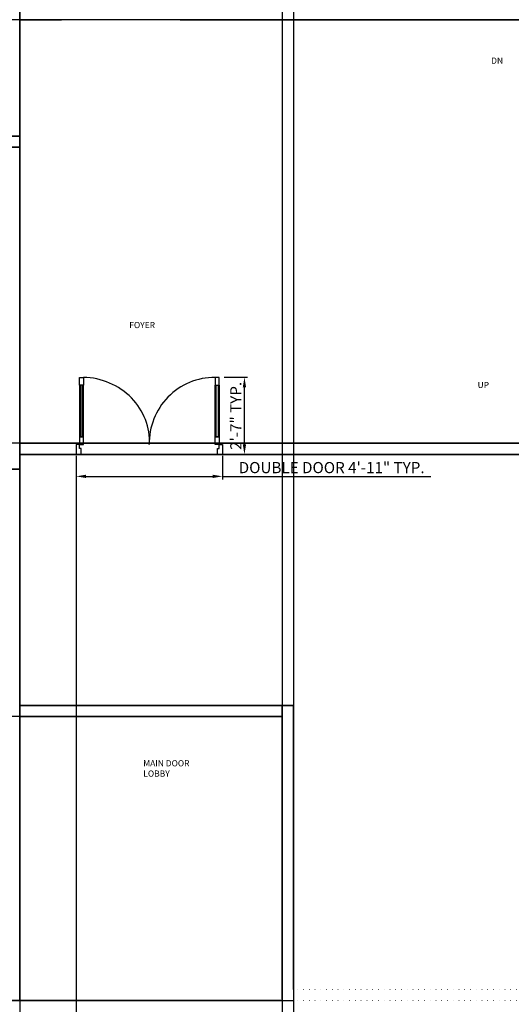
# Model space of a CAD drawing. Units: inches. Extents: x 1239 to 2276906, y 2273 to 321338.
# Tile 11 of 23: x 1556 to 1754, y 2629 to 3026. Entities that reach past the tile are written whole.
import ezdxf

# ---------------------------------------------------------------- set-up
doc = ezdxf.new("R2010")
doc.units = ezdxf.units.IN
doc.linetypes.add('DOT', pattern=[6.35, 0, -6.35])
for name, color, linetype, lineweight in [('A-ANNO-DIMS', 2, 'Continuous', 18), ('A-ANNO-TEXT', 7, 'Continuous', 18), ('A-AREA-IDEN', 7, 'Continuous', 18), ('A-FLOR-PORCH', 7, 'Continuous', 25), ('BEAM LINE', 4, 'DOT', 18), ('DOOR', 1, 'Continuous', 25), ('wall', 7, 'Continuous', 35)]:
    doc.layers.add(name, color=color, linetype=linetype, lineweight=lineweight)
doc.styles.get("Standard").update_dxf_attribs({"font": 'arial.ttf'})
doc.dimstyles.new('ISO-25', dxfattribs={"dimtxt": 4.5, "dimasz": 4, "dimexe": 1.25, "dimexo": 0.625, "dimtad": 1, "dimdec": 1, "dimlunit": 3, "dimtxsty": 'Standard', "dimcen": 2.5, "dimadec": 0, "dimazin": 0, "dimtfac": 1, "dimtdec": 1, "dimtmove": 0, "dimatfit": 3, "dimfxl": 1, "dimarcsym": 0})

# ---------------------------------------------------------------- blocks, each defined once
blk = doc.blocks.new('DOOR-DOUBLE-60')
for p, q in [((1.38, 27.95), (1.38, 31.1)), ((1.38, 31.1), (2.95, 31.1)), ((1.38, 27.95), (1.38, 7.09)), ((2.95, 27.95), (1.38, 27.95)), ((2.95, 27.95), (1.38, 27.95)), ((1.77, 27.95), (1.77, 7.09)), ((2.56, 27.95), (1.77, 27.95)), ((2.56, 7.09), (2.56, 27.95)), ((2.95, 31.1), (2.95, 27.95)), ((2.95, 7.09), (2.95, 27.95)), ((56.1, 31.1), (56.1, 27.95)), ((57.68, 31.1), (56.1, 31.1)), ((56.1, 27.95), (57.68, 27.95)), ((56.1, 7.09), (56.1, 27.95)), ((56.1, 27.95), (57.68, 27.95)), ((56.5, 7.09), (56.5, 27.95)), ((56.5, 27.95), (57.28, 27.95)), ((57.28, 27.95), (57.28, 7.09)), ((57.68, 27.95), (57.68, 31.1)), ((57.68, 27.95), (57.68, 7.09)), ((1.38, 7.09), (1.38, 3.94)), ((2.95, 7.09), (1.38, 7.09)), ((1.38, 7.09), (2.95, 7.09)), ((1.77, 7.09), (2.56, 7.09)), ((2.95, 3.94), (2.95, 7.09)), ((57.68, 7.09), (56.1, 7.09)), ((56.1, 3.94), (56.1, 7.09)), ((56.1, 7.09), (57.68, 7.09)), ((57.28, 7.09), (56.5, 7.09)), ((57.68, 7.09), (57.68, 3.94)), ((0, 3.94), (0, 0)), ((1.38, 3.94), (0, 3.94)), ((0, 0), (1.97, 0)), ((1.38, 3.94), (2.95, 3.94)), ((1.38, 2.36), (1.38, 3.94)), ((1.97, 2.36), (1.38, 2.36)), ((1.97, 1.97), (1.97, 2.36)), ((1.97, 0), (1.97, 1.97)), ((57.68, 3.94), (56.1, 3.94)), ((57.09, 1.97), (57.09, 2.36)), ((57.09, 2.36), (57.68, 2.36)), ((57.09, 0), (57.09, 1.97)), ((59.06, 0), (57.09, 0)), ((57.68, 3.94), (59.06, 3.94)), ((57.68, 2.36), (57.68, 3.94)), ((59.06, 3.94), (59.06, 0))]:
    blk.add_line(p, q)
blk.add_arc((55.99, 4.6), 26.5, 89.7657, 181.4438)
blk.add_ellipse((2.91, 5.95), major_axis=(26.26, -4.79), ratio=0.940794, start_param=0.11153, end_param=1.73917)
blk = doc.blocks.new('*D52')
at = {"layer": 'A-ANNO-DIMS', "color": 0, "lineweight": -2, "transparency": 16777216}
for p, q in [((1578.7, 2850.27), (1578.7, 2840.79)), ((1637.76, 2850.27), (1637.76, 2840.79)), ((1582.7, 2842.04), (1633.76, 2842.04)), ((1637.76, 2842.04), (1721.91, 2842.04))]:
    blk.add_line(p, q, dxfattribs=at)
at = {"layer": 'A-ANNO-DIMS', "color": 0, "transparency": 16777216}
for points in [[(1582.7, 2842.71), (1582.7, 2841.37), (1578.7, 2842.04)], [(1633.76, 2842.71), (1633.76, 2841.37), (1637.76, 2842.04)]]:
    blk.add_solid(points, dxfattribs=at)
at = {"layer": 'Defpoints', "color": 0, "transparency": 16777216}
for p in [(1578.7, 2850.9), (1637.76, 2850.9), (1637.76, 2842.04)]:
    blk.add_point(p, dxfattribs=at)
at = {"layer": 'A-ANNO-DIMS', "color": 0, "transparency": 16777216, "insert": (1681.83, 2844.99), "char_height": 4.5, "attachment_point": 5}
blk.add_mtext('DOUBLE DOOR 4\'-11" TYP.', dxfattribs=at)
blk = doc.blocks.new('*D53')
at = {"layer": 'A-ANNO-DIMS', "color": 0, "lineweight": -2, "transparency": 16777216}
for p, q in [((1638.38, 2882.03), (1647.86, 2882.03)), ((1646.61, 2854.9), (1646.61, 2878.03)), ((1638.38, 2850.9), (1647.86, 2850.9))]:
    blk.add_line(p, q, dxfattribs=at)
at = {"layer": 'A-ANNO-DIMS', "color": 0, "transparency": 16777216}
for points in [[(1645.95, 2878.03), (1647.28, 2878.03), (1646.61, 2882.03)], [(1645.95, 2854.9), (1647.28, 2854.9), (1646.61, 2850.9)]]:
    blk.add_solid(points, dxfattribs=at)
at = {"layer": 'Defpoints', "color": 0, "transparency": 16777216}
for p in [(1637.76, 2882.03), (1646.61, 2882.03), (1637.76, 2850.9)]:
    blk.add_point(p, dxfattribs=at)
at = {"layer": 'A-ANNO-DIMS', "color": 0, "transparency": 16777216, "insert": (1643.73, 2866.46), "char_height": 4.5, "attachment_point": 5, "rotation": 90}
blk.add_mtext('2\'-7" TYP.', dxfattribs=at)
blk = doc.blocks.new('*D87')
at = {"layer": 'A-ANNO-DIMS', "color": 0, "lineweight": -2, "transparency": 16777216}
for p, q in [((1666.38, 3250.77), (1666.38, 2275.7)), ((1921.38, 3250.77), (1921.38, 2275.7)), ((1670.38, 2276.95), (1917.38, 2276.95))]:
    blk.add_line(p, q, dxfattribs=at)
at = {"layer": 'A-ANNO-DIMS', "color": 0, "transparency": 16777216}
for points in [[(1670.38, 2277.61), (1670.38, 2276.28), (1666.38, 2276.95)], [(1917.38, 2277.61), (1917.38, 2276.28), (1921.38, 2276.95)]]:
    blk.add_solid(points, dxfattribs=at)
at = {"layer": 'Defpoints', "color": 0, "transparency": 16777216}
for p in [(1666.38, 3251.4), (1921.38, 3251.4), (1921.38, 2276.95)]:
    blk.add_point(p, dxfattribs=at)
at = {"layer": 'A-ANNO-DIMS', "color": 0, "transparency": 16777216, "insert": (1793.88, 2279.87), "char_height": 4.5, "attachment_point": 5}
blk.add_mtext('21\'-3"', dxfattribs=at)
blk = doc.blocks.new('*D96')
at = {"layer": 'A-ANNO-DIMS', "color": 0, "lineweight": -2, "transparency": 16777216}
for p, q in [((1555.88, 2629.77), (1555.88, 2275.7)), ((1661.88, 2629.77), (1661.88, 2275.7)), ((1559.88, 2276.95), (1657.88, 2276.95))]:
    blk.add_line(p, q, dxfattribs=at)
at = {"layer": 'A-ANNO-DIMS', "color": 0, "transparency": 16777216}
for points in [[(1559.88, 2277.61), (1559.88, 2276.28), (1555.88, 2276.95)], [(1657.88, 2277.61), (1657.88, 2276.28), (1661.88, 2276.95)]]:
    blk.add_solid(points, dxfattribs=at)
at = {"layer": 'Defpoints', "color": 0, "transparency": 16777216}
for p in [(1555.88, 2630.4), (1661.88, 2630.4), (1661.88, 2276.95)]:
    blk.add_point(p, dxfattribs=at)
at = {"layer": 'A-ANNO-DIMS', "color": 0, "transparency": 16777216, "insert": (1608.88, 2279.87), "char_height": 4.5, "attachment_point": 5}
blk.add_mtext('8\'-10"', dxfattribs=at)
blk = doc.blocks.new('*D97')
at = {"layer": 'A-ANNO-DIMS', "color": 0, "lineweight": -2, "transparency": 16777216}
for p, q in [((1661.26, 2745.04), (1247.33, 2745.04)), ((1248.58, 2634.4), (1248.58, 2741.04)), ((1661.26, 2630.4), (1247.33, 2630.4))]:
    blk.add_line(p, q, dxfattribs=at)
at = {"layer": 'A-ANNO-DIMS', "color": 0, "transparency": 16777216}
for points in [[(1247.92, 2741.04), (1249.25, 2741.04), (1248.58, 2745.04)], [(1247.92, 2634.4), (1249.25, 2634.4), (1248.58, 2630.4)]]:
    blk.add_solid(points, dxfattribs=at)
at = {"layer": 'Defpoints', "color": 0, "transparency": 16777216}
for p in [(1248.58, 2745.04), (1661.88, 2745.04), (1661.88, 2630.4)]:
    blk.add_point(p, dxfattribs=at)
at = {"layer": 'A-ANNO-DIMS', "color": 0, "transparency": 16777216, "insert": (1245.63, 2687.72), "char_height": 4.5, "attachment_point": 5, "rotation": 90}
blk.add_mtext('9\'-6 1/2"', dxfattribs=at)
blk = doc.blocks.new('*D98')
at = {"layer": 'A-ANNO-DIMS', "color": 0, "lineweight": -2, "transparency": 16777216}
for p, q in [((1772.76, 3026.4), (1247.33, 3026.4)), ((1248.58, 2859.4), (1248.58, 3022.4)), ((1772.76, 2855.4), (1247.33, 2855.4))]:
    blk.add_line(p, q, dxfattribs=at)
at = {"layer": 'A-ANNO-DIMS', "color": 0, "transparency": 16777216}
for points in [[(1247.92, 3022.4), (1249.25, 3022.4), (1248.58, 3026.4)], [(1247.92, 2859.4), (1249.25, 2859.4), (1248.58, 2855.4)]]:
    blk.add_solid(points, dxfattribs=at)
at = {"layer": 'Defpoints', "color": 0, "transparency": 16777216}
for p in [(1248.58, 3026.4), (1773.38, 3026.4), (1773.38, 2855.4)]:
    blk.add_point(p, dxfattribs=at)
at = {"layer": 'A-ANNO-DIMS', "color": 0, "transparency": 16777216, "insert": (1245.66, 2940.9), "char_height": 4.5, "attachment_point": 5, "rotation": 90}
blk.add_mtext('14\'-3"', dxfattribs=at)
blk = doc.blocks.new('*D111')
at = {"layer": 'A-ANNO-DIMS', "color": 0, "lineweight": -2, "transparency": 16777216}
for p, q in [((1547.38, 3607.7), (1543.38, 3607.7)), ((1551.38, 2635.52), (1551.38, 3608.95)), ((1551.38, 3607.7), (1555.88, 3607.7)), ((1555.88, 2631.02), (1555.88, 3608.95)), ((1559.88, 3607.7), (1587.58, 3607.7))]:
    blk.add_line(p, q, dxfattribs=at)
at = {"layer": 'A-ANNO-DIMS', "color": 0, "transparency": 16777216}
for points in [[(1547.38, 3608.36), (1547.38, 3607.03), (1551.38, 3607.7)], [(1559.88, 3608.36), (1559.88, 3607.03), (1555.88, 3607.7)]]:
    blk.add_solid(points, dxfattribs=at)
at = {"layer": 'Defpoints', "color": 0, "transparency": 16777216}
for p in [(1555.88, 3607.7), (1551.38, 2634.9), (1555.88, 2630.4)]:
    blk.add_point(p, dxfattribs=at)
at = {"layer": 'A-ANNO-DIMS', "color": 0, "transparency": 16777216, "insert": (1575.73, 3610.65), "char_height": 4.5, "attachment_point": 5}
blk.add_mtext('0\'-4 1/2"', dxfattribs=at)
blk = doc.blocks.new('*D112')
at = {"layer": 'A-ANNO-DIMS', "color": 0, "lineweight": -2, "transparency": 16777216}
for p, q in [((1555.88, 3371.77), (1555.88, 2275.7)), ((1661.88, 3371.77), (1661.88, 2275.7)), ((1559.88, 2276.95), (1657.88, 2276.95))]:
    blk.add_line(p, q, dxfattribs=at)
at = {"layer": 'A-ANNO-DIMS', "color": 0, "transparency": 16777216}
for points in [[(1559.88, 2277.61), (1559.88, 2276.28), (1555.88, 2276.95)], [(1657.88, 2277.61), (1657.88, 2276.28), (1661.88, 2276.95)]]:
    blk.add_solid(points, dxfattribs=at)
at = {"layer": 'Defpoints', "color": 0, "transparency": 16777216}
for p in [(1555.88, 3372.4), (1661.88, 3372.4), (1661.88, 2276.95)]:
    blk.add_point(p, dxfattribs=at)
at = {"layer": 'A-ANNO-DIMS', "color": 0, "transparency": 16777216, "insert": (1608.88, 2279.87), "char_height": 4.5, "attachment_point": 5}
blk.add_mtext('8\'-10"', dxfattribs=at)
blk = doc.blocks.new('*D114')
at = {"layer": 'A-ANNO-DIMS', "color": 0, "lineweight": -2, "transparency": 16777216}
for p, q in [((1555.88, 2850.27), (1555.88, 2275.7)), ((1578.7, 2850.27), (1578.7, 2275.7)), ((1559.88, 2276.95), (1574.7, 2276.95))]:
    blk.add_line(p, q, dxfattribs=at)
at = {"layer": 'A-ANNO-DIMS', "color": 0, "transparency": 16777216}
for points in [[(1559.88, 2277.61), (1559.88, 2276.28), (1555.88, 2276.95)], [(1574.7, 2277.61), (1574.7, 2276.28), (1578.7, 2276.95)]]:
    blk.add_solid(points, dxfattribs=at)
at = {"layer": 'Defpoints', "color": 0, "transparency": 16777216}
for p in [(1555.88, 2850.9), (1578.7, 2850.9), (1578.7, 2276.95)]:
    blk.add_point(p, dxfattribs=at)
at = {"layer": 'A-ANNO-DIMS', "color": 0, "transparency": 16777216, "insert": (1567.29, 2279.83), "char_height": 4.5, "attachment_point": 5}
blk.add_mtext('1\'-11"', dxfattribs=at)

msp = doc.modelspace()

# ---------------------------------------------------------------- linework, layer by layer
at = {"layer": 'A-FLOR-PORCH'}
msp.add_lwpolyline([(1551.38, 2630.4), (1666.38, 2630.4), (1666.38, 2555.13), (1551.38, 2555.13)], close=True, dxfattribs=at)
at = {"layer": 'BEAM LINE', "ltscale": 0.35}
for p, q in [((1921.38, 2634.9), (1666.38, 2634.9)), ((1921.38, 2630.4), (1661.88, 2630.4))]:
    msp.add_line(p, q, dxfattribs=at)
at = {"layer": 'wall'}
for p, q in [((1555.88, 3069.4), (1555.88, 2855.4)), ((1572.71, 3026.4), (1555.88, 3026.4)), ((1773.38, 3026.4), (1620.71, 3026.4)), ((1555.88, 2979.4), (1359.38, 2979.4)), ((1555.88, 2974.9), (1359.38, 2974.9)), ((1773.38, 2855.4), (1555.88, 2855.4)), ((1921.38, 2855.4), (1666.38, 2855.4)), ((1661.88, 2850.9), (1555.88, 2850.9)), ((1555.88, 2850.9), (1555.88, 2630.4)), ((1661.88, 2850.9), (1666.38, 2850.9)), ((1921.38, 2850.9), (1666.38, 2850.9)), ((1555.88, 2844.9), (1551.38, 2844.9)), ((1661.88, 2749.54), (1555.88, 2749.54)), ((1661.88, 2749.54), (1661.88, 2630.4)), ((1661.88, 2749.54), (1666.38, 2749.54)), ((1666.38, 2749.54), (1666.38, 2634.9)), ((1661.88, 2745.04), (1555.88, 2745.04)), ((1555.88, 2630.4), (1359.38, 2630.4))]:
    msp.add_line(p, q, dxfattribs=at)

# ---------------------------------------------------------------- block references
at = {"layer": 'DOOR'}
msp.add_blockref('DOOR-DOUBLE-60', (1578.7, 2850.9), dxfattribs=at)

# ---------------------------------------------------------------- texts
at = {"layer": 'A-ANNO-TEXT', "char_height": 2.5, "attachment_point": 1}
for s, insert in [('DN ', (1746.22, 3011.12)), ('UP', (1740.74, 2880.18))]:
    msp.add_mtext_dynamic_manual_height_columns(s, width=44.9462, gutter_width=12.5, heights=[0], dxfattribs=dict(at, insert=insert))
at = {"layer": 'A-AREA-IDEN', "char_height": 2.5, "attachment_point": 1}
for s, insert in [('FOYER', (1600.12, 2904.38)), ('MAIN DOOR\\PLOBBY', (1605.79, 2727.46))]:
    msp.add_mtext_dynamic_manual_height_columns(s, width=44.9462, gutter_width=12.5, heights=[0], dxfattribs=dict(at, insert=insert))

# ---------------------------------------------------------------- dimensions: what is measured, and where the dimension line sits
at = {"layer": 'A-ANNO-DIMS'}
for base, p1, p2, picture, middle in [((1555.88, 3607.7), (1551.38, 2634.9), (1555.88, 2630.4), '*D111', (1575.73, 3610.65)), ((1661.88, 2276.95), (1555.88, 3372.4), (1661.88, 3372.4), '*D112', (1608.88, 2279.87)), ((1921.38, 2276.95), (1666.38, 3251.4), (1921.38, 3251.4), '*D87', (1793.88, 2279.87)), ((1578.7, 2276.95), (1555.88, 2850.9), (1578.7, 2850.9), '*D114', (1567.29, 2279.83)), ((1661.88, 2276.95), (1555.88, 2630.4), (1661.88, 2630.4), '*D96', (1608.88, 2279.87))]:
    dim = msp.add_linear_dim(base=base, p1=p1, p2=p2, dimstyle='ISO-25', override={"dimdec": 1, "dimlfac": 1, "dimrnd": 0, "dimzin": 1, "dimdsep": 46, "dimlunit": 4, "dimfrac": 2}, dxfattribs=at)
    dim.commit()
    dim.dimension.update_dxf_attribs({"geometry": picture, "text_midpoint": middle})
for base, p1, p2, picture, middle in [((1248.58, 3026.4), (1773.38, 2855.4), (1773.38, 3026.4), '*D98', (1245.66, 2940.9)), ((1248.58, 2745.04), (1661.88, 2630.4), (1661.88, 2745.04), '*D97', (1245.63, 2687.72))]:
    dim = msp.add_linear_dim(base=base, p1=p1, p2=p2, angle=90, dimstyle='ISO-25', override={"dimdec": 1, "dimlfac": 1, "dimrnd": 0, "dimzin": 1, "dimdsep": 46, "dimlunit": 4, "dimfrac": 2}, dxfattribs=at)
    dim.commit()
    dim.dimension.update_dxf_attribs({"geometry": picture, "text_midpoint": middle})
dim = msp.add_linear_dim(base=(1646.61, 2882.03), p1=(1637.76, 2850.9), p2=(1637.76, 2882.03), angle=90, text='<> TYP.', dimstyle='ISO-25', override={"dimdec": 1, "dimlfac": 1, "dimrnd": 0, "dimzin": 1, "dimdsep": 46, "dimlunit": 4, "dimfrac": 2}, dxfattribs=at)
dim.commit()
dim.dimension.update_dxf_attribs({"geometry": '*D53', "text_midpoint": (1643.73, 2866.46)})
dim = msp.add_linear_dim(base=(1637.76, 2842.04), p1=(1578.7, 2850.9), p2=(1637.76, 2850.9), text='DOUBLE DOOR <> TYP.', dimstyle='ISO-25', override={"dimdec": 1, "dimlfac": 1, "dimrnd": 0, "dimzin": 1, "dimdsep": 46, "dimlunit": 4, "dimfrac": 2}, dxfattribs=at)
dim.commit()
dim.dimension.update_dxf_attribs({"geometry": '*D52', "text_midpoint": (1681.83, 2844.99)})

doc.saveas('drawing.dxf')
